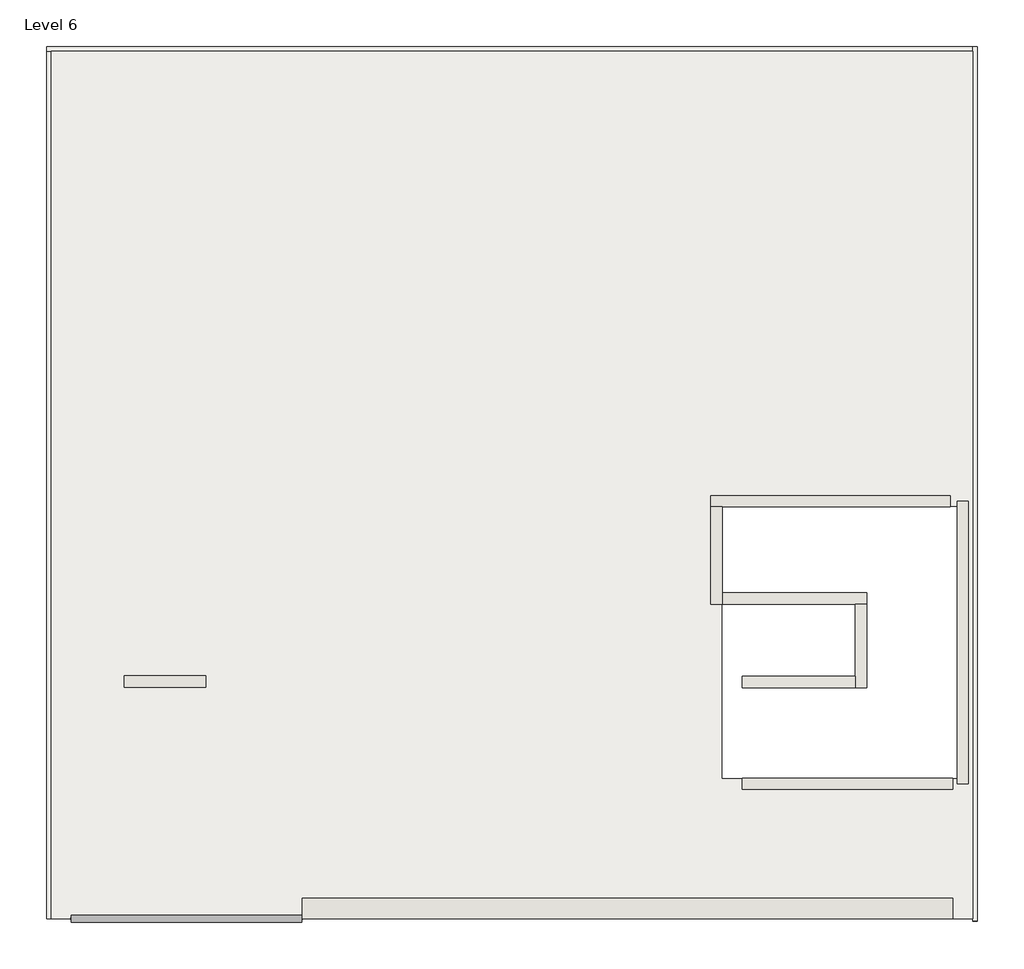
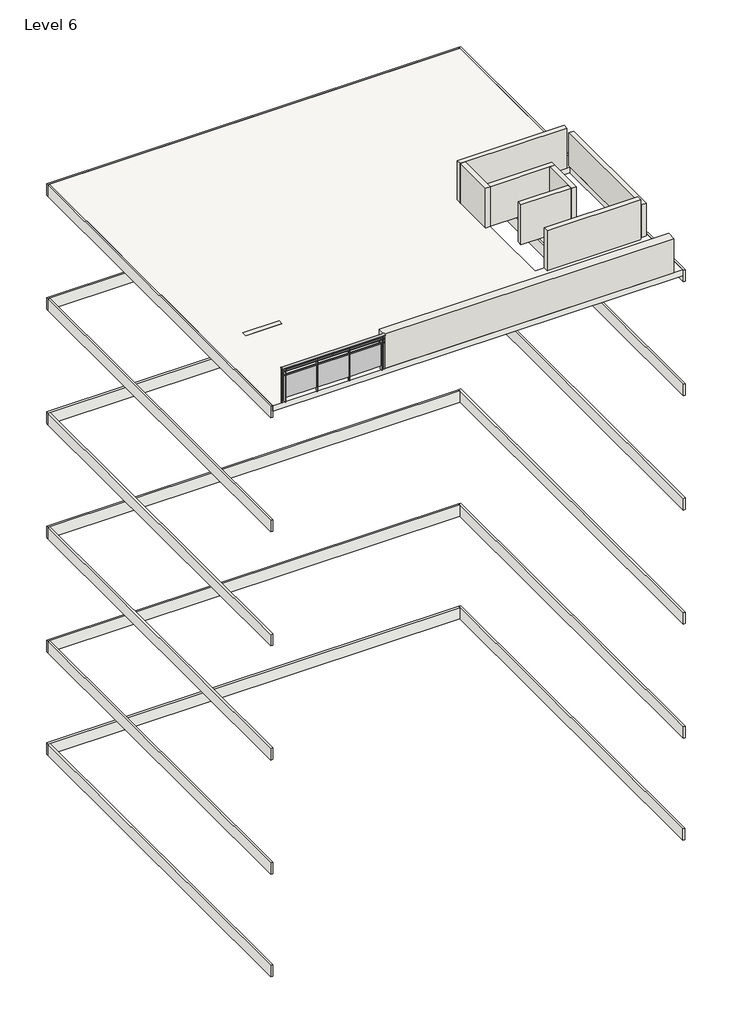
# One storey: 9 walls, 2 slabs, 1 railing.
"""IFC4 building model written with IfcOpenShell, lengths in millimetres."""

from ifc_helpers import new_model, si_unit, point, frame, origin, place, context, project, spatial, polyline, ellipse_curve, trimmed, outline, extrude, faceted_brep, transform, mapped, element, save
from ifc_brep_helpers import plane_surface, extruded_surface, advanced_brep
from components import floors_1_floors_1_bc35289f

model = new_model("IFC4")

# Units and contexts
model_context = context("Model", 3, world=origin())
ifc_project = project(units=[si_unit("LENGTHUNIT", "METRE", prefix="MILLI")], contexts=[model_context])

# Site, building, storey
site = spatial("IfcSite", under=ifc_project)
building = spatial("IfcBuilding", under=site)
storey = spatial("IfcBuildingStorey", under=building, Name="Level 6", Elevation=15240.0)

# Railing
placement = place(None, origin())
element("IfcRailing", 1, ObjectType="Glass Panel - Bottom Fill", at=placement, inside=storey, context=model_context, shape_type="SolidModel", body=[
    advanced_brep(
    [(-6296.2569651, 489.6055142, 16154.4), (-6296.2569651, 413.4055142, 16154.4), (-3705.4569651, 489.6055142, 16154.4), (-3705.4569651, 413.4055142, 16154.4)],
    [
        (0, 1, ellipse_curve(frame((-6296.2569651, 451.5055142, 16154.4), z_axis=(-1.0, 0.0, 0.0), x_axis=(0.0, -1.0, 0.0)), 38.1, 28.575)),
        (1, 0, ellipse_curve(frame((-6296.2569651, 451.5055142, 16154.4), z_axis=(-1.0, 0.0, 0.0), x_axis=(0.0, -1.0, 0.0)), 38.1, 28.575)),
        (2, 3, ellipse_curve(frame((-3705.4569651, 451.5055142, 16154.4), z_axis=(1.0, 0.0, 0.0), x_axis=(0.0, -1.0, 0.0)), 38.1, 28.575)),
        (3, 2, ellipse_curve(frame((-3705.4569651, 451.5055142, 16154.4), z_axis=(1.0, 0.0, 0.0), x_axis=(0.0, -1.0, 0.0)), 38.1, 28.575)),
        (0, 2),
        (3, 1),
    ],
    [
        plane_surface(frame((-6296.2569651, 451.5055142, 16154.4), z_axis=(-1.0, 0.0, 0.0), x_axis=(0.0, 1.0, 0.0))),
        plane_surface(frame((-3705.4569651, 451.5055142, 16154.4), z_axis=(1.0, 0.0, 0.0), x_axis=(0.0, 1.0, 0.0))),
        extruded_surface(trimmed(ellipse_curve(frame((-3705.4569651, 451.5055142, 16154.4), z_axis=(-1.0, 0.0, 0.0), x_axis=(0.0, -1.0, 0.0)), 38.1, 28.575), [point((-3705.4569651, 489.6055142, 16154.4))], [point((-3705.4569651, 413.4055142, 16154.4))], True, "CARTESIAN"), (-2590.8, 0.0, 0.0), 2590.8),
        extruded_surface(trimmed(ellipse_curve(frame((-3705.4569651, 451.5055142, 16154.4), z_axis=(-1.0, 0.0, 0.0), x_axis=(0.0, -1.0, 0.0)), 38.1, 28.575), [point((-3705.4569651, 413.4055142, 16154.4))], [point((-3705.4569651, 489.6055142, 16154.4))], True, "CARTESIAN"), (-2590.8, 0.0, 0.0), 2590.8),
    ],
    [
        (0, [[1, 2]]),
        (1, [[3, 4]]),
        (2, [[-1, 5, -4, 6]]),
        (3, [[-2, -6, -3, -5]]),
    ],
),
    extrude(outline(polyline([(-6296.2569651, 438.8055142), (-6296.2569651, 464.2055142), (-3705.4569651, 464.2055142), (-3705.4569651, 438.8055142), (-6296.2569651, 438.8055142)])), frame((0.0, 0.0, 16040.1), z_axis=(0.0, 0.0, 1.0), x_axis=(1.0, 0.0, 0.0)), (0.0, 0.0, 1.0), 25.4),
    extrude(outline(polyline([(-6296.2569651, 438.8055142), (-6296.2569651, 464.2055142), (-3705.4569651, 464.2055142), (-3705.4569651, 438.8055142), (-6296.2569651, 438.8055142)])), frame((0.0, 0.0, 15938.5), z_axis=(0.0, 0.0, 1.0), x_axis=(1.0, 0.0, 0.0)), (0.0, 0.0, 1.0), 25.4),
    extrude(outline(polyline([(-3788.0069651, 426.1055142), (-3788.0069651, 476.9055142), (-3775.3069651, 476.9055142), (-3775.3069651, 426.1055142), (-3788.0069651, 426.1055142)])), frame((0.0, 0.0, 15240.0), z_axis=(0.0, 0.0, 1.0), x_axis=(1.0, 0.0, 0.0)), (0.0, 0.0, 1.0), 885.6788223),
    extrude(outline(polyline([(-4594.4569651, 458.0406712), (-3781.6569651, 458.0406712), (-3781.6569651, 451.6906712), (-4594.4569651, 451.6906712), (-4594.4569651, 458.0406712)])), frame((0.0, 0.0, 15341.6), z_axis=(0.0, 0.0, 1.0), x_axis=(1.0, 0.0, 0.0)), (0.0, 0.0, 1.0), 596.9),
    extrude(outline(polyline([(-4600.8069651, 426.1055142), (-4600.8069651, 476.9055142), (-4588.1069651, 476.9055142), (-4588.1069651, 426.1055142), (-4600.8069651, 426.1055142)])), frame((0.0, 0.0, 15240.0), z_axis=(0.0, 0.0, 1.0), x_axis=(1.0, 0.0, 0.0)), (0.0, 0.0, 1.0), 885.6788223),
    extrude(outline(polyline([(-5407.2569651, 458.0406712), (-4594.4569651, 458.0406712), (-4594.4569651, 451.6906712), (-5407.2569651, 451.6906712), (-5407.2569651, 458.0406712)])), frame((0.0, 0.0, 15341.6), z_axis=(0.0, 0.0, 1.0), x_axis=(1.0, 0.0, 0.0)), (0.0, 0.0, 1.0), 596.9),
    extrude(outline(polyline([(-5413.6069651, 426.1055142), (-5413.6069651, 476.9055142), (-5400.9069651, 476.9055142), (-5400.9069651, 426.1055142), (-5413.6069651, 426.1055142)])), frame((0.0, 0.0, 15240.0), z_axis=(0.0, 0.0, 1.0), x_axis=(1.0, 0.0, 0.0)), (0.0, 0.0, 1.0), 885.6788223),
    extrude(outline(polyline([(-6220.0569651, 458.0406712), (-5407.2569651, 458.0406712), (-5407.2569651, 451.6906712), (-6220.0569651, 451.6906712), (-6220.0569651, 458.0406712)])), frame((0.0, 0.0, 15341.6), z_axis=(0.0, 0.0, 1.0), x_axis=(1.0, 0.0, 0.0)), (0.0, 0.0, 1.0), 596.9),
    extrude(outline(polyline([(-6226.4069651, 426.1055142), (-6226.4069651, 476.9055142), (-6213.7069651, 476.9055142), (-6213.7069651, 426.1055142), (-6226.4069651, 426.1055142)])), frame((0.0, 0.0, 15240.0), z_axis=(0.0, 0.0, 1.0), x_axis=(1.0, 0.0, 0.0)), (0.0, 0.0, 1.0), 885.6788223),
    extrude(outline(polyline([(-3718.1569651, 441.9805142), (-3718.1569651, 461.0305142), (-3699.1069651, 461.0305142), (-3699.1069651, 441.9805142), (-3718.1569651, 441.9805142)])), frame((0.0, 0.0, 15240.0), z_axis=(0.0, 0.0, 1.0), x_axis=(1.0, 0.0, 0.0)), (0.0, 0.0, 1.0), 885.6788223),
    extrude(outline(polyline([(-6302.6069651, 441.9805142), (-6302.6069651, 461.0305142), (-6283.5569651, 461.0305142), (-6283.5569651, 441.9805142), (-6302.6069651, 441.9805142)])), frame((0.0, 0.0, 15240.0), z_axis=(0.0, 0.0, 1.0), x_axis=(1.0, 0.0, 0.0)), (0.0, 0.0, 1.0), 885.6788223),
])

# Slabs
floors_1_floors_1_shape = floors_1_floors_1_bc35289f(model_context)
element("IfcSlab", 2, ObjectType="Floors 1 : Floors 1", at=placement, inside=storey, context=model_context, shape_type="MappedRepresentation", body=[
    mapped(floors_1_floors_1_shape, transform((0.0, 0.0, 0.0), x_axis=(1.0, 0.0, 0.0), y_axis=(0.0, 1.0, 0.0), z_axis=(0.0, 0.0, 1.0))),
])
element("IfcSlab", 3, ObjectType="Generic - 12\"", at=placement, inside=storey, context=model_context, shape_type="SweptSolid", body=[
    extrude(outline(polyline([(3838.3430349, 10205.1055142), (3838.3430349, 451.5055142), (-6524.8569651, 451.5055142), (-6524.8569651, 10205.1055142), (3838.3430349, 10205.1055142)]), holes=[polyline([(3660.5430349, 5080.6555142), (1018.9430349, 5080.6555142), (1018.9430349, 2032.6555142), (3660.5430349, 2032.6555142), (3660.5430349, 5080.6555142)])]), frame((0.0, 0.0, 15087.6), z_axis=(0.0, 0.0, 1.0), x_axis=(1.0, 0.0, 0.0)), (0.0, 0.0, 1.0), 152.4),
])

# Walls
element("IfcWall", 4, ObjectType="5\"", at=placement, inside=storey, context=model_context, shape_type="Brep", body=[
    faceted_brep([(3584.3430349, 5207.6555142, 15240.0), (891.9430349, 5207.6555142, 15240.0), (891.9430349, 5207.6555142, 16306.8), (3584.3430349, 5207.6555142, 16306.8), (3584.3430349, 5080.6555142, 15240.0), (3584.3430349, 5080.6555142, 16306.8), (1018.9430349, 5080.6555142, 16306.8), (891.9430349, 5080.6555142, 16306.8), (891.9430349, 5080.6555142, 15240.0), (1018.9430349, 5080.6555142, 15240.0)], [[[0, 1, 2, 3]], [[4, 5, 6, 7, 8, 9]], [[2, 1, 8, 7]], [[1, 0, 4, 9, 8]], [[3, 2, 7, 6, 5]], [[0, 3, 5, 4]]]),
])
element("IfcWall", 5, ObjectType="5\"", at=placement, inside=storey, context=model_context, shape_type="Brep", body=[
    faceted_brep([(891.9430349, 5080.6555142, 15240.0), (891.9430349, 3988.4555142, 15240.0), (891.9430349, 3988.4555142, 16306.8), (891.9430349, 5080.6555142, 16306.8), (1018.9430349, 5080.6555142, 15240.0), (1018.9430349, 5080.6555142, 16306.8), (1018.9430349, 4115.4555142, 16306.8), (1018.9430349, 3988.4555142, 16306.8), (1018.9430349, 3988.4555142, 15240.0), (1018.9430349, 4115.4555142, 15240.0)], [[[0, 1, 2, 3]], [[4, 5, 6, 7, 8, 9]], [[1, 0, 4, 9, 8]], [[3, 2, 7, 6, 5]], [[0, 3, 5, 4]], [[2, 1, 8, 7]]]),
])
element("IfcWall", 6, ObjectType="5\"", at=placement, inside=storey, context=model_context, shape_type="Brep", body=[
    faceted_brep([(1018.9430349, 3988.4555142, 15240.0), (2517.5430349, 3988.4555142, 15240.0), (2644.5430349, 3988.4555142, 15240.0), (2644.5430349, 3988.4555142, 16306.8), (2517.5430349, 3988.4555142, 16306.8), (1018.9430349, 3988.4555142, 16306.8), (1018.9430349, 4115.4555142, 15240.0), (1018.9430349, 4115.4555142, 16306.8), (2644.5430349, 4115.4555142, 16306.8), (2644.5430349, 4115.4555142, 15240.0)], [[[0, 1, 2, 3, 4, 5]], [[6, 7, 8, 9]], [[2, 1, 0, 6, 9]], [[5, 4, 3, 8, 7]], [[0, 5, 7, 6]], [[3, 2, 9, 8]]]),
])
element("IfcWall", 7, ObjectType="5\"", at=placement, inside=storey, context=model_context, shape_type="Brep", body=[
    faceted_brep([(2517.5430349, 3988.4555142, 15240.0), (2517.5430349, 3175.6555142, 15240.0), (2517.5430349, 3048.6555142, 15240.0), (2517.5430349, 3048.6555142, 16306.8), (2517.5430349, 3175.6555142, 16306.8), (2517.5430349, 3988.4555142, 16306.8), (2644.5430349, 3988.4555142, 15240.0), (2644.5430349, 3988.4555142, 16306.8), (2644.5430349, 3048.6555142, 16306.8), (2644.5430349, 3048.6555142, 15240.0)], [[[0, 1, 2, 3, 4, 5]], [[6, 7, 8, 9]], [[2, 1, 0, 6, 9]], [[5, 4, 3, 8, 7]], [[0, 5, 7, 6]], [[3, 2, 9, 8]]]),
])
element("IfcWall", 8, ObjectType="5\"", at=placement, inside=storey, context=model_context, shape_type="SweptSolid", body=[
    extrude(outline(polyline([(1247.5430349, 3175.6555142), (2517.5430349, 3175.6555142), (2517.5430349, 3048.6555142), (1247.5430349, 3048.6555142), (1247.5430349, 3175.6555142)])), frame((0.0, 0.0, 15240.0), z_axis=(0.0, 0.0, 1.0), x_axis=(1.0, 0.0, 0.0)), (0.0, 0.0, 1.0), 1066.8),
])
element("IfcWall", 9, ObjectType="5\"", at=placement, inside=storey, context=model_context, shape_type="SweptSolid", body=[
    extrude(outline(polyline([(3609.7430349, 1905.6555142), (1247.5430349, 1905.6555142), (1247.5430349, 2032.6555142), (3609.7430349, 2032.6555142), (3609.7430349, 1905.6555142)])), frame((0.0, 0.0, 15240.0), z_axis=(0.0, 0.0, 1.0), x_axis=(1.0, 0.0, 0.0)), (0.0, 0.0, 1.0), 1066.8),
])
element("IfcWall", 10, ObjectType="5\"", at=placement, inside=storey, context=model_context, shape_type="SweptSolid", body=[
    extrude(outline(polyline([(3787.5430349, 5144.1555142), (3787.5430349, 1969.1555142), (3660.5430349, 1969.1555142), (3660.5430349, 5144.1555142), (3787.5430349, 5144.1555142)])), frame((0.0, 0.0, 15240.0), z_axis=(0.0, 0.0, 1.0), x_axis=(1.0, 0.0, 0.0)), (0.0, 0.0, 1.0), 876.3),
])
element("IfcWall", 11, ObjectType="5\"", at=placement, inside=storey, context=model_context, shape_type="SweptSolid", body=[
    extrude(outline(polyline([(-4784.9569651, 3055.0055142), (-5699.3569651, 3055.0055142), (-5699.3569651, 3182.0055142), (-4784.9569651, 3182.0055142), (-4784.9569651, 3055.0055142)])), frame((0.0, 0.0, 14300.2), z_axis=(0.0, 0.0, 1.0), x_axis=(1.0, 0.0, 0.0)), (0.0, 0.0, 1.0), 939.8),
])
element("IfcWall", 12, ObjectType="9\"", at=placement, inside=storey, context=model_context, shape_type="Brep", body=[
    faceted_brep([(3609.7430349, 680.1055142, 15240.0), (-3699.1069651, 680.1055142, 15240.0), (-3699.1069651, 680.1055142, 16154.4), (3609.7430349, 680.1055142, 16154.4), (3609.7430349, 451.5055142, 15240.0), (3609.7430349, 451.5055142, 16154.4), (-3699.1069651, 451.5055142, 16154.4), (-3699.1069651, 451.5055142, 15240.0), (3609.7430349, 578.5055142, 15240.0)], [[[0, 1, 2, 3]], [[4, 5, 6, 7]], [[0, 3, 5, 4, 8]], [[1, 0, 8, 4, 7]], [[2, 1, 7, 6]], [[3, 2, 6, 5]]]),
])

save(model, "model.ifc")

# Revit data of these elements
# Type "Glass Panel - Bottom Fill"
#   Assembly Code = "C2010400"
#   built-in parameter 1008612 = 0.0416667 (stored number, unit not read)
#   built-in parameter 1008611 = 0.0416667 (stored number, unit not read)
#   built-in parameter 1008609 = 0.333333 (stored number, unit not read)
#   built-in parameter 1008604 = 0.166667 (stored number, unit not read)
#   built-in parameter 1008603 = 0.166667 (stored number, unit not read)
#   Railing Height = 3' - 0"
#   built-in parameter 1008630 = 2
#   built-in parameter 1008610 = 2
#   built-in parameter 1008618 = Baluster - Square : 3/4"
# Type "Generic - 12\""
#   Assembly Code = "B1010"
#   Function = 0
#   Layers, outside or top first: 0' - 6" no material (function 1)
# Type "5\""
#   Assembly Code = "B2010"
#   Layers, outside or top first: 0' - 5" "Concrete Masonry Units" (function 1)
# Type "9\""
#   Assembly Code = "B2010"
#   Layers, outside or top first: 0' - 9" no material (function 1)
# Element 1 (IfcRailing, "Glass Panel - Bottom Fill")
#   Phase Created = New Construction
#   Materials on its faces: "Glass"
# Element 2 (IfcSlab, "Floors 1 : Floors 1")
#   Phase Created = New Construction
#   Materials on its faces: "1 wall brown", "Default Floor"
# Element 3 (IfcSlab, "Generic - 12\"")
#   Height Offset From Level = 0' - 0"
#   Phase Created = New Construction
#   Materials on its faces: "Default Floor", "1 wall brown"
# Elements 4, 5, 7, 8 (IfcWall, "5\"")
#   Top Offset = 0' - 0"
#   Base Offset = 0' - 0"
#   Unconnected Height = 3' - 6"
#   wall height = 3' - 6"
#   Phase Created = New Construction
#   Base Constraint = Level 6
#   Materials on its faces: "Concrete Masonry Units", "1 wall white"
# Elements 6, 9 (IfcWall, "5\"")
#   Top Offset = 0' - 0"
#   Base Offset = 0' - 0"
#   Unconnected Height = 3' - 6"
#   wall height = 3' - 6"
#   Phase Created = New Construction
#   Base Constraint = Level 6
#   Materials on its faces: "1 wall white", "Concrete Masonry Units"
# Element 10 (IfcWall, "5\"")
#   Top Offset = 0' - 0"
#   Base Offset = 0' - 0"
#   Unconnected Height = 3' - 0"
#   wall height = 3' - 0"
#   Phase Created = New Construction
#   Base Constraint = Level 6
#   Materials on its faces: "Concrete Masonry Units"
# Element 11 (IfcWall, "5\"")
#   built-in parameter 1001111 = -3' - 1"
#   Top Offset = 0' - 0"
#   Base Offset = -3' - 1"
#   Unconnected Height = 3' - 1"
#   wall height = 3' - 1"
#   Phase Created = New Construction
#   Base Constraint = Level 6
#   Materials on its faces: "Concrete Masonry Units", "1 wall white"
# Element 12 (IfcWall, "9\"")
#   Top Offset = 0' - 0"
#   Base Offset = 0' - 0"
#   Unconnected Height = 3' - 0"
#   wall height = 3' - 0"
#   Phase Created = New Construction
#   Base Constraint = Level 6
#   Materials on its faces: "1 wall white", "Default Wall"
# Materials
#   "Concrete Masonry Units": class "Masonry", colour RGB 227 227 227, transparency 0, Description = "Concrete masonry units", Cost = 0
#   "Glass": class "Glass", colour RGB 0 128 192, transparency 0.75, Description = "Soda Lime Glass", Cost = 0
#   "1 wall brown": class "Generic", colour RGB 61 46 37, transparency 0, Cost = 0
#   "Default Floor": colour RGB 128 128 128, transparency 0, Cost = 0
#   "1 wall white": class "Generic", colour RGB 244 245 241, transparency 0, Cost = 0
#   "Default Wall": colour RGB 128 128 128, transparency 0, Cost = 0
